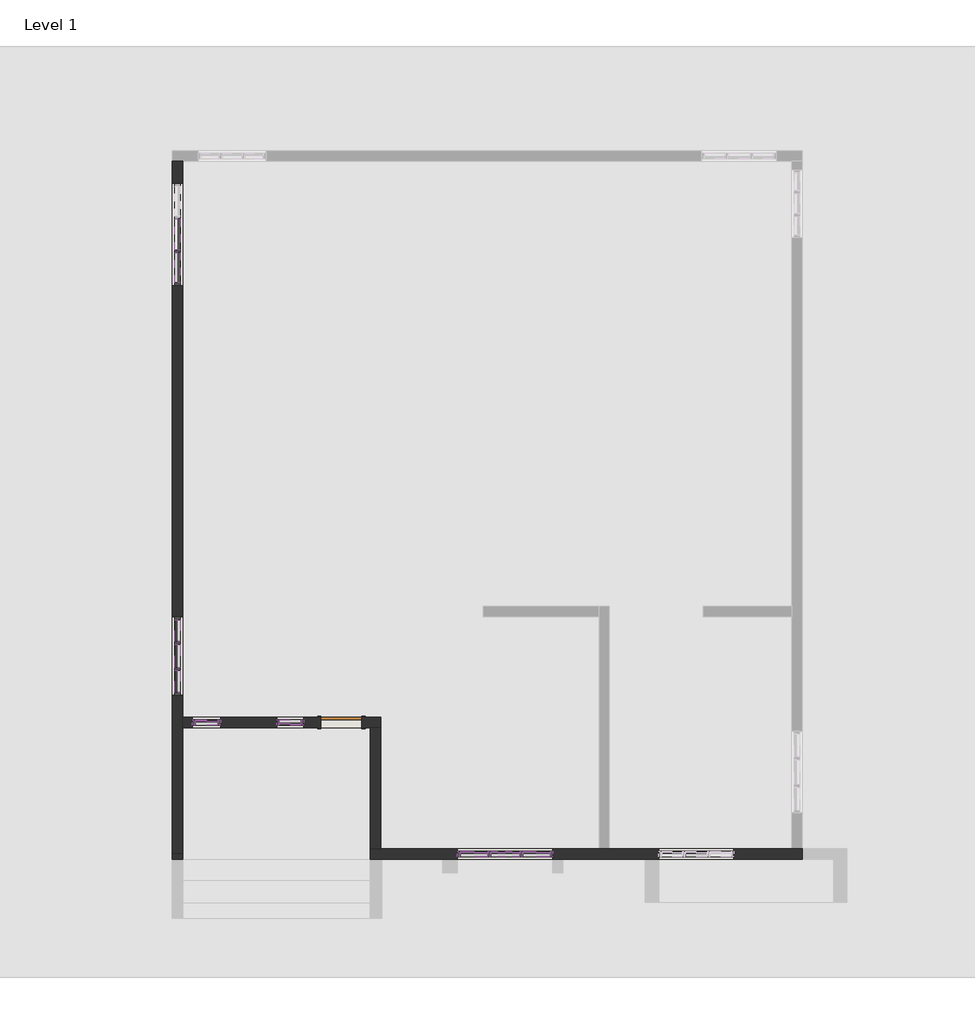
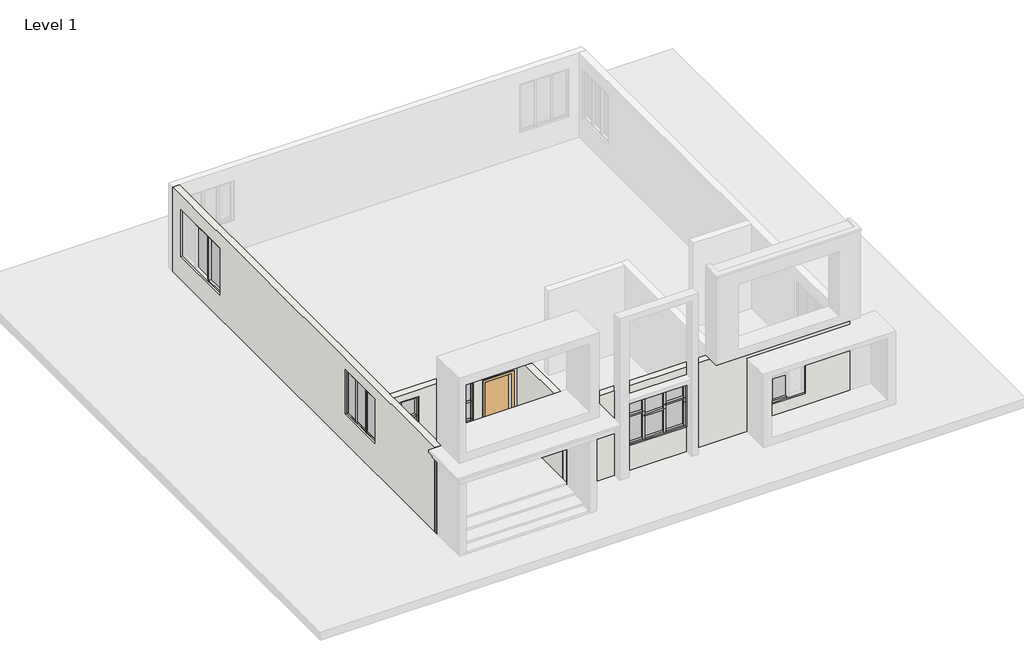
# One storey, part 1 of 2: 59 members, 19 plates, 5 walls, 1 door.
"""IFC4 building model written with IfcOpenShell, lengths in millimetres."""

from ifc_helpers import new_model, si_unit, origin, origin_with_axes, place, context, project, spatial, polyline, outline, extrude, faceted_brep, transform, mapped, element, save
from components import door_0ca8825f, member_5535eeb3, member_2ebf4a73, member_b955a9e9, member_c33c434a, member_d74592ed, member_67d70a96, member_b9f3750b, member_8f80d2aa, member_96e46165, member_de9b0c97, member_7fd687a9, member_90750a43, member_a9816f27, member_b70ee1cc, member_323df77c, member_86d06fe4, member_8600bbed, member_e53b78c9, member_5215b92c, member_3f0e0172, member_1cc7c027, member_f6f0dfdd, member_f8dc38bf, member_47c7a801, member_876f8f00, member_f09d9db7, member_ac493aea, member_2944fbe8, system_panel_glazed_7de79e50, system_panel_glazed_57682dc0, system_panel_glazed_8ac636d5, system_panel_glazed_c23b727d, system_panel_glazed_e55ceb02, system_panel_glazed_b26b014f, system_panel_glazed_bdd26bb3, system_panel_glazed_e612b4c2, system_panel_glazed_0ac8c76b, system_panel_glazed_a09e93fe, system_panel_glazed_b9962699, system_panel_glazed_c7c048a3, system_panel_glazed_0ee6699b, system_panel_glazed_40386fdd, system_panel_glazed_3330f8c4

model = new_model("IFC4")

# Units and contexts
model_context = context("Model", 3, world=origin())
ifc_project = project(units=[si_unit("LENGTHUNIT", "METRE", prefix="MILLI")], contexts=[model_context])

# Site, building, storey
site = spatial("IfcSite", under=ifc_project)
building = spatial("IfcBuilding", under=site)
storey = spatial("IfcBuildingStorey", under=building, Name="Level 1", Elevation=0.0)

# Door
placement = place(None, origin())
door_shape = door_0ca8825f(model_context)
element("IfcDoor", 1, ObjectType="Single-Flush : 36\" x 84\"", at=placement, inside=storey, context=model_context, shape_type="MappedRepresentation", body=[
    mapped(door_shape, transform((-18079.9097681, -11198.7339922, 406.4), x_axis=(1.0, 0.0, 0.0), y_axis=(0.0, 1.0, 0.0), z_axis=(0.0, 0.0, 1.0))),
])

# Members
member_shape = member_5535eeb3(model_context)
element("IfcMember", 2, ObjectType="Rectangular Mullion : 2.5\" x 5\" rectangular", at=placement, inside=storey, context=model_context, shape_type="MappedRepresentation", body=[
    mapped(member_shape, transform((-10466.2597681, -14132.4339922, 2463.7993261), x_axis=(0.0, 0.0, 1.0), y_axis=(0.0, -1.0, 0.0), z_axis=(1.0, 0.0, 0.0))),
])
member_2_shape = member_2ebf4a73(model_context)
element("IfcMember", 3, ObjectType="Rectangular Mullion : 2.5\" x 5\" rectangular", at=placement, inside=storey, context=model_context, shape_type="MappedRepresentation", body=[
    mapped(member_2_shape, transform((-10402.7597681, -14132.4339922, 684.1737808), x_axis=(0.0, 0.0, -1.0), y_axis=(0.0, -1.0, 0.0), z_axis=(-1.0, 0.0, 0.0))),
])
member_3_shape = member_b955a9e9(model_context)
element("IfcMember", 4, ObjectType="Rectangular Mullion : 2.5\" x 5\" rectangular", at=placement, inside=storey, context=model_context, shape_type="MappedRepresentation", body=[
    mapped(member_3_shape, transform((-21737.5097681, -651.3839922, 2530.4981779), x_axis=(0.0, 0.0, 1.0), y_axis=(-1.0, 0.0, 0.0), z_axis=(0.0, -1.0, 0.0))),
])
member_4_shape = member_c33c434a(model_context)
element("IfcMember", 5, ObjectType="Rectangular Mullion : 2.5\" x 5\" rectangular", at=placement, inside=storey, context=model_context, shape_type="MappedRepresentation", body=[
    mapped(member_4_shape, transform((-21737.5097681, -1381.6339922, 2530.4981779), x_axis=(0.0, 0.0, 1.0), y_axis=(-1.0, 0.0, 0.0), z_axis=(0.0, -1.0, 0.0))),
])
member_5_shape = member_d74592ed(model_context)
element("IfcMember", 6, ObjectType="Rectangular Mullion : 2.5\" x 5\" rectangular", at=placement, inside=storey, context=model_context, shape_type="MappedRepresentation", body=[
    mapped(member_5_shape, transform((-21737.5097681, -683.1339922, 850.000156), x_axis=(0.0, -1.0, 0.0), y_axis=(-1.0, 0.0, 0.0), z_axis=(0.0, 0.0, -1.0))),
])
element("IfcMember", 7, ObjectType="Rectangular Mullion : 2.5\" x 5\" rectangular", at=placement, inside=storey, context=model_context, shape_type="MappedRepresentation", body=[
    mapped(member_4_shape, transform((-21737.5097681, -714.8839922, 850.000156), x_axis=(0.0, 0.0, -1.0), y_axis=(-1.0, 0.0, 0.0), z_axis=(0.0, 1.0, 0.0))),
])
member_6_shape = member_67d70a96(model_context)
element("IfcMember", 8, ObjectType="Rectangular Mullion : 2.5\" x 5\" rectangular", at=placement, inside=storey, context=model_context, shape_type="MappedRepresentation", body=[
    mapped(member_6_shape, transform((-21737.5097681, -1445.1339922, 850.000156), x_axis=(0.0, -1.0, 0.0), y_axis=(-1.0, 0.0, 0.0), z_axis=(0.0, 0.0, -1.0))),
])
member_7_shape = member_b9f3750b(model_context)
element("IfcMember", 9, ObjectType="Rectangular Mullion : 2.5\" x 5\" rectangular", at=placement, inside=storey, context=model_context, shape_type="MappedRepresentation", body=[
    mapped(member_7_shape, transform((-21737.5097681, -10036.6839922, 2655.4428848), x_axis=(0.0, 0.0, 1.0), y_axis=(1.0, 0.0, 0.0), z_axis=(0.0, 1.0, 0.0))),
])
element("IfcMember", 10, ObjectType="Rectangular Mullion : 2.5\" x 5\" rectangular", at=placement, inside=storey, context=model_context, shape_type="MappedRepresentation", body=[
    mapped(member_7_shape, transform((-21737.5097681, -8900.0339922, 2655.4428848), x_axis=(0.0, 0.0, 1.0), y_axis=(1.0, 0.0, 0.0), z_axis=(0.0, 1.0, 0.0))),
])
member_8_shape = member_8f80d2aa(model_context)
element("IfcMember", 11, ObjectType="Rectangular Mullion : 2.5\" x 5\" rectangular", at=placement, inside=storey, context=model_context, shape_type="MappedRepresentation", body=[
    mapped(member_8_shape, transform((-21737.5097681, -9452.4839922, 2655.4428848), x_axis=(0.0, 0.0, 1.0), y_axis=(1.0, 0.0, 0.0), z_axis=(0.0, 1.0, 0.0))),
])
member_9_shape = member_96e46165(model_context)
element("IfcMember", 12, ObjectType="Rectangular Mullion : 2.5\" x 5\" rectangular", at=placement, inside=storey, context=model_context, shape_type="MappedRepresentation", body=[
    mapped(member_9_shape, transform((-21737.5097681, -9420.7339922, 1049.1745099), x_axis=(0.0, 1.0, 0.0), y_axis=(1.0, 0.0, 0.0), z_axis=(0.0, 0.0, -1.0))),
])
element("IfcMember", 13, ObjectType="Rectangular Mullion : 2.5\" x 5\" rectangular", at=placement, inside=storey, context=model_context, shape_type="MappedRepresentation", body=[
    mapped(member_9_shape, transform((-21737.5097681, -10004.9339922, 1049.1745099), x_axis=(0.0, 1.0, 0.0), y_axis=(1.0, 0.0, 0.0), z_axis=(0.0, 0.0, -1.0))),
])
element("IfcMember", 14, ObjectType="Rectangular Mullion : 2.5\" x 5\" rectangular", at=placement, inside=storey, context=model_context, shape_type="MappedRepresentation", body=[
    mapped(member_8_shape, transform((-21737.5097681, -9973.1839922, 1049.1745099), x_axis=(0.0, 0.0, -1.0), y_axis=(1.0, 0.0, 0.0), z_axis=(0.0, -1.0, 0.0))),
])
element("IfcMember", 15, ObjectType="Rectangular Mullion : 2.5\" x 5\" rectangular", at=placement, inside=storey, context=model_context, shape_type="MappedRepresentation", body=[
    mapped(member_7_shape, transform((-21737.5097681, -9388.9839922, 1049.1745099), x_axis=(0.0, 0.0, -1.0), y_axis=(1.0, 0.0, 0.0), z_axis=(0.0, -1.0, 0.0))),
])
element("IfcMember", 16, ObjectType="Rectangular Mullion : 2.5\" x 5\" rectangular", at=placement, inside=storey, context=model_context, shape_type="MappedRepresentation", body=[
    mapped(member_7_shape, transform((-21737.5097681, -10525.6339922, 1049.1745099), x_axis=(0.0, 0.0, -1.0), y_axis=(1.0, 0.0, 0.0), z_axis=(0.0, -1.0, 0.0))),
])
member_10_shape = member_de9b0c97(model_context)
element("IfcMember", 17, ObjectType="Rectangular Mullion : 2.5\" x 5\" rectangular", at=placement, inside=storey, context=model_context, shape_type="MappedRepresentation", body=[
    mapped(member_10_shape, transform((-21737.5097681, -10589.1339922, 2655.4428848), x_axis=(0.0, -1.0, 0.0), y_axis=(1.0, 0.0, 0.0), z_axis=(0.0, 0.0, 1.0))),
])
element("IfcMember", 18, ObjectType="Rectangular Mullion : 2.5\" x 5\" rectangular", at=placement, inside=storey, context=model_context, shape_type="MappedRepresentation", body=[
    mapped(member_10_shape, transform((-21737.5097681, -8836.5339922, 1049.1745099), x_axis=(0.0, 1.0, 0.0), y_axis=(1.0, 0.0, 0.0), z_axis=(0.0, 0.0, -1.0))),
])
member_11_shape = member_7fd687a9(model_context)
element("IfcMember", 19, ObjectType="Rectangular Mullion : 2.5\" x 5\" rectangular", at=placement, inside=storey, context=model_context, shape_type="MappedRepresentation", body=[
    mapped(member_11_shape, transform((-20835.8097681, -11198.7339922, 2808.8134726), x_axis=(0.0, 0.0, 1.0), y_axis=(0.0, -1.0, 0.0), z_axis=(1.0, 0.0, 0.0))),
])
member_12_shape = member_90750a43(model_context)
element("IfcMember", 20, ObjectType="Rectangular Mullion : 2.5\" x 5\" rectangular", at=placement, inside=storey, context=model_context, shape_type="MappedRepresentation", body=[
    mapped(member_12_shape, transform((-20835.8097681, -11198.7339922, 2112.2396553), x_axis=(0.0, 0.0, 1.0), y_axis=(0.0, -1.0, 0.0), z_axis=(1.0, 0.0, 0.0))),
])
element("IfcMember", 21, ObjectType="Rectangular Mullion : 2.5\" x 5\" rectangular", at=placement, inside=storey, context=model_context, shape_type="MappedRepresentation", body=[
    mapped(member_12_shape, transform((-20835.8097681, -11198.7339922, 1415.6658381), x_axis=(0.0, 0.0, 1.0), y_axis=(0.0, -1.0, 0.0), z_axis=(1.0, 0.0, 0.0))),
])
member_13_shape = member_a9816f27(model_context)
element("IfcMember", 22, ObjectType="Rectangular Mullion : 2.5\" x 5\" rectangular", at=placement, inside=storey, context=model_context, shape_type="MappedRepresentation", body=[
    mapped(member_13_shape, transform((-20772.3097681, -11198.7339922, 2112.2396553), x_axis=(1.0, 0.0, 0.0), y_axis=(0.0, -1.0, 0.0), z_axis=(0.0, 0.0, -1.0))),
])
element("IfcMember", 23, ObjectType="Rectangular Mullion : 2.5\" x 5\" rectangular", at=placement, inside=storey, context=model_context, shape_type="MappedRepresentation", body=[
    mapped(member_13_shape, transform((-21407.3097681, -11198.7339922, 2808.8134726), x_axis=(-1.0, 0.0, 0.0), y_axis=(0.0, -1.0, 0.0), z_axis=(0.0, 0.0, 1.0))),
])
element("IfcMember", 24, ObjectType="Rectangular Mullion : 2.5\" x 5\" rectangular", at=placement, inside=storey, context=model_context, shape_type="MappedRepresentation", body=[
    mapped(member_13_shape, transform((-20772.3097681, -11198.7339922, 1415.6658381), x_axis=(1.0, 0.0, 0.0), y_axis=(0.0, -1.0, 0.0), z_axis=(0.0, 0.0, -1.0))),
])
element("IfcMember", 25, ObjectType="Rectangular Mullion : 2.5\" x 5\" rectangular", at=placement, inside=storey, context=model_context, shape_type="MappedRepresentation", body=[
    mapped(member_13_shape, transform((-21407.3097681, -11198.7339922, 2112.2396553), x_axis=(-1.0, 0.0, 0.0), y_axis=(0.0, -1.0, 0.0), z_axis=(0.0, 0.0, 1.0))),
])
element("IfcMember", 26, ObjectType="Rectangular Mullion : 2.5\" x 5\" rectangular", at=placement, inside=storey, context=model_context, shape_type="MappedRepresentation", body=[
    mapped(member_11_shape, transform((-21343.8097681, -11198.7339922, 719.0920209), x_axis=(0.0, 0.0, -1.0), y_axis=(0.0, -1.0, 0.0), z_axis=(-1.0, 0.0, 0.0))),
])
element("IfcMember", 27, ObjectType="Rectangular Mullion : 2.5\" x 5\" rectangular", at=placement, inside=storey, context=model_context, shape_type="MappedRepresentation", body=[
    mapped(member_13_shape, transform((-20772.3097681, -11198.7339922, 719.0920209), x_axis=(1.0, 0.0, 0.0), y_axis=(0.0, -1.0, 0.0), z_axis=(0.0, 0.0, -1.0))),
])
element("IfcMember", 28, ObjectType="Rectangular Mullion : 2.5\" x 5\" rectangular", at=placement, inside=storey, context=model_context, shape_type="MappedRepresentation", body=[
    mapped(member_13_shape, transform((-21407.3097681, -11198.7339922, 1415.6658381), x_axis=(-1.0, 0.0, 0.0), y_axis=(0.0, -1.0, 0.0), z_axis=(0.0, 0.0, 1.0))),
])
member_14_shape = member_b70ee1cc(model_context)
element("IfcMember", 29, ObjectType="Rectangular Mullion : 2.5\" x 5\" rectangular", at=placement, inside=storey, context=model_context, shape_type="MappedRepresentation", body=[
    mapped(member_14_shape, transform((-19527.7097681, -11198.7339922, 1978.8215035), x_axis=(-1.0, 0.0, 0.0), y_axis=(0.0, 1.0, 0.0), z_axis=(0.0, 0.0, -1.0))),
])
member_15_shape = member_323df77c(model_context)
element("IfcMember", 30, ObjectType="Rectangular Mullion : 2.5\" x 5\" rectangular", at=placement, inside=storey, context=model_context, shape_type="MappedRepresentation", body=[
    mapped(member_15_shape, transform((-19464.2097681, -11198.7339922, 1978.8215035), x_axis=(0.0, 0.0, 1.0), y_axis=(0.0, 1.0, 0.0), z_axis=(-1.0, 0.0, 0.0))),
])
element("IfcMember", 31, ObjectType="Rectangular Mullion : 2.5\" x 5\" rectangular", at=placement, inside=storey, context=model_context, shape_type="MappedRepresentation", body=[
    mapped(member_15_shape, transform((-19464.2097681, -11198.7339922, 1330.4078609), x_axis=(0.0, 0.0, 1.0), y_axis=(0.0, 1.0, 0.0), z_axis=(-1.0, 0.0, 0.0))),
])
member_16_shape = member_86d06fe4(model_context)
element("IfcMember", 32, ObjectType="Rectangular Mullion : 2.5\" x 5\" rectangular", at=placement, inside=storey, context=model_context, shape_type="MappedRepresentation", body=[
    mapped(member_16_shape, transform((-19464.2097681, -11198.7339922, 2842.4215035), x_axis=(0.0, 0.0, 1.0), y_axis=(0.0, 1.0, 0.0), z_axis=(-1.0, 0.0, 0.0))),
])
element("IfcMember", 33, ObjectType="Rectangular Mullion : 2.5\" x 5\" rectangular", at=placement, inside=storey, context=model_context, shape_type="MappedRepresentation", body=[
    mapped(member_14_shape, transform((-18918.1097681, -11198.7339922, 2842.4215035), x_axis=(1.0, 0.0, 0.0), y_axis=(0.0, 1.0, 0.0), z_axis=(0.0, 0.0, 1.0))),
])
element("IfcMember", 34, ObjectType="Rectangular Mullion : 2.5\" x 5\" rectangular", at=placement, inside=storey, context=model_context, shape_type="MappedRepresentation", body=[
    mapped(member_16_shape, transform((-18981.6097681, -11198.7339922, 681.9942183), x_axis=(0.0, 0.0, -1.0), y_axis=(0.0, 1.0, 0.0), z_axis=(1.0, 0.0, 0.0))),
])
member_17_shape = member_8600bbed(model_context)
element("IfcMember", 35, ObjectType="Rectangular Mullion : 2.5\" x 5\" rectangular", at=placement, inside=storey, context=model_context, shape_type="MappedRepresentation", body=[
    mapped(member_17_shape, transform((-19527.7097681, -11198.7339922, 1330.4078609), x_axis=(-1.0, 0.0, 0.0), y_axis=(0.0, 1.0, 0.0), z_axis=(0.0, 0.0, -1.0))),
])
element("IfcMember", 36, ObjectType="Rectangular Mullion : 2.5\" x 5\" rectangular", at=placement, inside=storey, context=model_context, shape_type="MappedRepresentation", body=[
    mapped(member_17_shape, transform((-19527.7097681, -11198.7339922, 681.9942183), x_axis=(-1.0, 0.0, 0.0), y_axis=(0.0, 1.0, 0.0), z_axis=(0.0, 0.0, -1.0))),
])
element("IfcMember", 37, ObjectType="Rectangular Mullion : 2.5\" x 5\" rectangular", at=placement, inside=storey, context=model_context, shape_type="MappedRepresentation", body=[
    mapped(member_17_shape, transform((-18918.1097681, -11198.7339922, 1330.4078609), x_axis=(1.0, 0.0, 0.0), y_axis=(0.0, 1.0, 0.0), z_axis=(0.0, 0.0, 1.0))),
])
element("IfcMember", 38, ObjectType="Rectangular Mullion : 2.5\" x 5\" rectangular", at=placement, inside=storey, context=model_context, shape_type="MappedRepresentation", body=[
    mapped(member_17_shape, transform((-18918.1097681, -11198.7339922, 1978.8215035), x_axis=(1.0, 0.0, 0.0), y_axis=(0.0, 1.0, 0.0), z_axis=(0.0, 0.0, 1.0))),
])
member_18_shape = member_e53b78c9(model_context)
element("IfcMember", 39, ObjectType="Rectangular Mullion : 2.5\" x 5\" rectangular", at=placement, inside=storey, context=model_context, shape_type="MappedRepresentation", body=[
    mapped(member_18_shape, transform((-14098.4597681, -14132.4339922, 1762.5660143), x_axis=(0.0, 0.0, 1.0), y_axis=(0.0, -1.0, 0.0), z_axis=(1.0, 0.0, 0.0))),
])
member_19_shape = member_5215b92c(model_context)
element("IfcMember", 40, ObjectType="Rectangular Mullion : 2.5\" x 5\" rectangular", at=placement, inside=storey, context=model_context, shape_type="MappedRepresentation", body=[
    mapped(member_19_shape, transform((-14098.4597681, -14132.4339922, 2636.1562178), x_axis=(0.0, 0.0, 1.0), y_axis=(0.0, -1.0, 0.0), z_axis=(1.0, 0.0, 0.0))),
])
member_20_shape = member_3f0e0172(model_context)
element("IfcMember", 41, ObjectType="Rectangular Mullion : 2.5\" x 5\" rectangular", at=placement, inside=storey, context=model_context, shape_type="MappedRepresentation", body=[
    mapped(member_20_shape, transform((-14809.6597681, -14132.4339922, 2636.1562178), x_axis=(0.0, 0.0, 1.0), y_axis=(0.0, -1.0, 0.0), z_axis=(1.0, 0.0, 0.0))),
])
element("IfcMember", 42, ObjectType="Rectangular Mullion : 2.5\" x 5\" rectangular", at=placement, inside=storey, context=model_context, shape_type="MappedRepresentation", body=[
    mapped(member_20_shape, transform((-13419.0097681, -14132.4339922, 2636.1562178), x_axis=(0.0, 0.0, 1.0), y_axis=(0.0, -1.0, 0.0), z_axis=(1.0, 0.0, 0.0))),
])
member_21_shape = member_1cc7c027(model_context)
element("IfcMember", 43, ObjectType="Rectangular Mullion : 2.5\" x 5\" rectangular", at=placement, inside=storey, context=model_context, shape_type="MappedRepresentation", body=[
    mapped(member_21_shape, transform((-14777.9097681, -14132.4339922, 1914.9660143), x_axis=(1.0, 0.0, 0.0), y_axis=(0.0, -1.0, 0.0), z_axis=(0.0, 0.0, -1.0))),
])
element("IfcMember", 44, ObjectType="Rectangular Mullion : 2.5\" x 5\" rectangular", at=placement, inside=storey, context=model_context, shape_type="MappedRepresentation", body=[
    mapped(member_21_shape, transform((-14066.7097681, -14132.4339922, 1914.9660143), x_axis=(1.0, 0.0, 0.0), y_axis=(0.0, -1.0, 0.0), z_axis=(0.0, 0.0, -1.0))),
])
member_22_shape = member_f6f0dfdd(model_context)
element("IfcMember", 45, ObjectType="Rectangular Mullion : 2.5\" x 5\" rectangular", at=placement, inside=storey, context=model_context, shape_type="MappedRepresentation", body=[
    mapped(member_22_shape, transform((-14777.9097681, -14132.4339922, 1762.5660143), x_axis=(1.0, 0.0, 0.0), y_axis=(0.0, -1.0, 0.0), z_axis=(0.0, 0.0, -1.0))),
])
element("IfcMember", 46, ObjectType="Rectangular Mullion : 2.5\" x 5\" rectangular", at=placement, inside=storey, context=model_context, shape_type="MappedRepresentation", body=[
    mapped(member_22_shape, transform((-14066.7097681, -14132.4339922, 1762.5660143), x_axis=(1.0, 0.0, 0.0), y_axis=(0.0, -1.0, 0.0), z_axis=(0.0, 0.0, -1.0))),
])
member_23_shape = member_f8dc38bf(model_context)
element("IfcMember", 47, ObjectType="Rectangular Mullion : 2.5\" x 5\" rectangular", at=placement, inside=storey, context=model_context, shape_type="MappedRepresentation", body=[
    mapped(member_23_shape, transform((-13419.0097681, -14132.4339922, 1914.9660143), x_axis=(0.0, 0.0, 1.0), y_axis=(0.0, -1.0, 0.0), z_axis=(1.0, 0.0, 0.0))),
])
element("IfcMember", 48, ObjectType="Rectangular Mullion : 2.5\" x 5\" rectangular", at=placement, inside=storey, context=model_context, shape_type="MappedRepresentation", body=[
    mapped(member_23_shape, transform((-14809.6597681, -14132.4339922, 1914.9660143), x_axis=(0.0, 0.0, 1.0), y_axis=(0.0, -1.0, 0.0), z_axis=(1.0, 0.0, 0.0))),
])
member_24_shape = member_47c7a801(model_context)
element("IfcMember", 49, ObjectType="Rectangular Mullion : 2.5\" x 5\" rectangular", at=placement, inside=storey, context=model_context, shape_type="MappedRepresentation", body=[
    mapped(member_24_shape, transform((-13355.5097681, -14132.4339922, 1914.9660143), x_axis=(1.0, 0.0, 0.0), y_axis=(0.0, -1.0, 0.0), z_axis=(0.0, 0.0, -1.0))),
])
member_25_shape = member_876f8f00(model_context)
element("IfcMember", 50, ObjectType="Rectangular Mullion : 2.5\" x 5\" rectangular", at=placement, inside=storey, context=model_context, shape_type="MappedRepresentation", body=[
    mapped(member_25_shape, transform((-13355.5097681, -14132.4339922, 1762.5660143), x_axis=(1.0, 0.0, 0.0), y_axis=(0.0, -1.0, 0.0), z_axis=(0.0, 0.0, -1.0))),
])
element("IfcMember", 51, ObjectType="Rectangular Mullion : 2.5\" x 5\" rectangular", at=placement, inside=storey, context=model_context, shape_type="MappedRepresentation", body=[
    mapped(member_25_shape, transform((-15489.1097681, -14132.4339922, 1914.9660143), x_axis=(-1.0, 0.0, 0.0), y_axis=(0.0, -1.0, 0.0), z_axis=(0.0, 0.0, 1.0))),
])
element("IfcMember", 52, ObjectType="Rectangular Mullion : 2.5\" x 5\" rectangular", at=placement, inside=storey, context=model_context, shape_type="MappedRepresentation", body=[
    mapped(member_24_shape, transform((-15489.1097681, -14132.4339922, 2636.1562178), x_axis=(-1.0, 0.0, 0.0), y_axis=(0.0, -1.0, 0.0), z_axis=(0.0, 0.0, 1.0))),
])
member_26_shape = member_f09d9db7(model_context)
element("IfcMember", 53, ObjectType="Rectangular Mullion : 2.5\" x 5\" rectangular", at=placement, inside=storey, context=model_context, shape_type="MappedRepresentation", body=[
    mapped(member_26_shape, transform((-14777.9097681, -14132.4339922, 888.9758108), x_axis=(1.0, 0.0, 0.0), y_axis=(0.0, -1.0, 0.0), z_axis=(0.0, 0.0, -1.0))),
])
element("IfcMember", 54, ObjectType="Rectangular Mullion : 2.5\" x 5\" rectangular", at=placement, inside=storey, context=model_context, shape_type="MappedRepresentation", body=[
    mapped(member_26_shape, transform((-14066.7097681, -14132.4339922, 888.9758108), x_axis=(1.0, 0.0, 0.0), y_axis=(0.0, -1.0, 0.0), z_axis=(0.0, 0.0, -1.0))),
])
element("IfcMember", 55, ObjectType="Rectangular Mullion : 2.5\" x 5\" rectangular", at=placement, inside=storey, context=model_context, shape_type="MappedRepresentation", body=[
    mapped(member_20_shape, transform((-14034.9597681, -14132.4339922, 888.9758108), x_axis=(0.0, 0.0, -1.0), y_axis=(0.0, -1.0, 0.0), z_axis=(-1.0, 0.0, 0.0))),
])
element("IfcMember", 56, ObjectType="Rectangular Mullion : 2.5\" x 5\" rectangular", at=placement, inside=storey, context=model_context, shape_type="MappedRepresentation", body=[
    mapped(member_20_shape, transform((-15425.6097681, -14132.4339922, 888.9758108), x_axis=(0.0, 0.0, -1.0), y_axis=(0.0, -1.0, 0.0), z_axis=(-1.0, 0.0, 0.0))),
])
element("IfcMember", 57, ObjectType="Rectangular Mullion : 2.5\" x 5\" rectangular", at=placement, inside=storey, context=model_context, shape_type="MappedRepresentation", body=[
    mapped(member_19_shape, transform((-14746.1597681, -14132.4339922, 888.9758108), x_axis=(0.0, 0.0, -1.0), y_axis=(0.0, -1.0, 0.0), z_axis=(-1.0, 0.0, 0.0))),
])
member_27_shape = member_ac493aea(model_context)
element("IfcMember", 58, ObjectType="Rectangular Mullion : 2.5\" x 5\" rectangular", at=placement, inside=storey, context=model_context, shape_type="MappedRepresentation", body=[
    mapped(member_27_shape, transform((-13355.5097681, -14132.4339922, 888.9758108), x_axis=(1.0, 0.0, 0.0), y_axis=(0.0, -1.0, 0.0), z_axis=(0.0, 0.0, -1.0))),
])
element("IfcMember", 59, ObjectType="Rectangular Mullion : 2.5\" x 5\" rectangular", at=placement, inside=storey, context=model_context, shape_type="MappedRepresentation", body=[
    mapped(member_27_shape, transform((-15489.1097681, -14132.4339922, 1762.5660143), x_axis=(-1.0, 0.0, 0.0), y_axis=(0.0, -1.0, 0.0), z_axis=(0.0, 0.0, 1.0))),
])
member_28_shape = member_2944fbe8(model_context)
element("IfcMember", 60, ObjectType="Rectangular Mullion : 2.5\" x 5\" rectangular", at=placement, inside=storey, context=model_context, shape_type="MappedRepresentation", body=[
    mapped(member_28_shape, transform((-10993.3097681, -14132.4339922, 2463.7993261), x_axis=(-1.0, 0.0, 0.0), y_axis=(0.0, -1.0, 0.0), z_axis=(0.0, 0.0, 1.0))),
])

# Plates
system_panel_glazed_shape = system_panel_glazed_7de79e50(model_context)
element("IfcPlate", 61, ObjectType="System Panel : Glazed", at=placement, inside=storey, context=model_context, shape_type="MappedRepresentation", body=[
    mapped(system_panel_glazed_shape, transform((-21737.5097681, -1048.2589922, 913.500156), x_axis=(0.0, -1.0, 0.0), y_axis=(1.0, 0.0, 0.0), z_axis=(0.0, 0.0, 1.0))),
])
system_panel_glazed_2_shape = system_panel_glazed_57682dc0(model_context)
element("IfcPlate", 62, ObjectType="System Panel : Glazed", at=placement, inside=storey, context=model_context, shape_type="MappedRepresentation", body=[
    mapped(system_panel_glazed_2_shape, transform((-21737.5097681, -302.1339922, 913.500156), x_axis=(0.0, -1.0, 0.0), y_axis=(1.0, 0.0, 0.0), z_axis=(0.0, 0.0, 1.0))),
])
system_panel_glazed_3_shape = system_panel_glazed_8ac636d5(model_context)
element("IfcPlate", 63, ObjectType="System Panel : Glazed", at=placement, inside=storey, context=model_context, shape_type="MappedRepresentation", body=[
    mapped(system_panel_glazed_3_shape, transform((-21737.5097681, -10281.1589922, 1112.6745099), x_axis=(0.0, 1.0, 0.0), y_axis=(-1.0, 0.0, 0.0), z_axis=(0.0, 0.0, 1.0))),
])
element("IfcPlate", 64, ObjectType="System Panel : Glazed", at=placement, inside=storey, context=model_context, shape_type="MappedRepresentation", body=[
    mapped(system_panel_glazed_3_shape, transform((-21737.5097681, -9144.5089922, 1112.6745099), x_axis=(0.0, 1.0, 0.0), y_axis=(-1.0, 0.0, 0.0), z_axis=(0.0, 0.0, 1.0))),
])
system_panel_glazed_4_shape = system_panel_glazed_c23b727d(model_context)
element("IfcPlate", 65, ObjectType="System Panel : Glazed", at=placement, inside=storey, context=model_context, shape_type="MappedRepresentation", body=[
    mapped(system_panel_glazed_4_shape, transform((-21737.5097681, -9712.8339922, 1112.6745099), x_axis=(0.0, 1.0, 0.0), y_axis=(-1.0, 0.0, 0.0), z_axis=(0.0, 0.0, 1.0))),
])
system_panel_glazed_5_shape = system_panel_glazed_e55ceb02(model_context)
element("IfcPlate", 66, ObjectType="System Panel : Glazed", at=placement, inside=storey, context=model_context, shape_type="MappedRepresentation", body=[
    mapped(system_panel_glazed_5_shape, transform((-21089.8097681, -11198.7339922, 782.5920209), x_axis=(1.0, 0.0, 0.0), y_axis=(0.0, 1.0, 0.0), z_axis=(0.0, 0.0, 1.0))),
])
element("IfcPlate", 67, ObjectType="System Panel : Glazed", at=placement, inside=storey, context=model_context, shape_type="MappedRepresentation", body=[
    mapped(system_panel_glazed_5_shape, transform((-21089.8097681, -11198.7339922, 2143.9896553), x_axis=(1.0, 0.0, 0.0), y_axis=(0.0, 1.0, 0.0), z_axis=(0.0, 0.0, 1.0))),
])
system_panel_glazed_6_shape = system_panel_glazed_b26b014f(model_context)
element("IfcPlate", 68, ObjectType="System Panel : Glazed", at=placement, inside=storey, context=model_context, shape_type="MappedRepresentation", body=[
    mapped(system_panel_glazed_6_shape, transform((-21089.8097681, -11198.7339922, 1447.4158381), x_axis=(1.0, 0.0, 0.0), y_axis=(0.0, 1.0, 0.0), z_axis=(0.0, 0.0, 1.0))),
])
system_panel_glazed_7_shape = system_panel_glazed_bdd26bb3(model_context)
element("IfcPlate", 69, ObjectType="System Panel : Glazed", at=placement, inside=storey, context=model_context, shape_type="MappedRepresentation", body=[
    mapped(system_panel_glazed_7_shape, transform((-19222.9097681, -11198.7339922, 2010.5715035), x_axis=(-1.0, 0.0, 0.0), y_axis=(0.0, -1.0, 0.0), z_axis=(0.0, 0.0, 1.0))),
])
system_panel_glazed_8_shape = system_panel_glazed_e612b4c2(model_context)
element("IfcPlate", 70, ObjectType="System Panel : Glazed", at=placement, inside=storey, context=model_context, shape_type="MappedRepresentation", body=[
    mapped(system_panel_glazed_8_shape, transform((-19222.9097681, -11198.7339922, 1362.1578609), x_axis=(-1.0, 0.0, 0.0), y_axis=(0.0, -1.0, 0.0), z_axis=(0.0, 0.0, 1.0))),
])
system_panel_glazed_9_shape = system_panel_glazed_0ac8c76b(model_context)
element("IfcPlate", 71, ObjectType="System Panel : Glazed", at=placement, inside=storey, context=model_context, shape_type="MappedRepresentation", body=[
    mapped(system_panel_glazed_9_shape, transform((-19222.9097681, -11198.7339922, 745.4942183), x_axis=(-1.0, 0.0, 0.0), y_axis=(0.0, -1.0, 0.0), z_axis=(0.0, 0.0, 1.0))),
])
system_panel_glazed_10_shape = system_panel_glazed_a09e93fe(model_context)
element("IfcPlate", 72, ObjectType="System Panel : Glazed", at=placement, inside=storey, context=model_context, shape_type="MappedRepresentation", body=[
    mapped(system_panel_glazed_10_shape, transform((-14422.3097681, -14132.4339922, 1794.3160143), x_axis=(1.0, 0.0, 0.0), y_axis=(0.0, 1.0, 0.0), z_axis=(0.0, 0.0, 1.0))),
])
system_panel_glazed_11_shape = system_panel_glazed_b9962699(model_context)
element("IfcPlate", 73, ObjectType="System Panel : Glazed", at=placement, inside=storey, context=model_context, shape_type="MappedRepresentation", body=[
    mapped(system_panel_glazed_11_shape, transform((-15117.6347681, -14132.4339922, 1946.7160143), x_axis=(1.0, 0.0, 0.0), y_axis=(0.0, 1.0, 0.0), z_axis=(0.0, 0.0, 1.0))),
])
element("IfcPlate", 74, ObjectType="System Panel : Glazed", at=placement, inside=storey, context=model_context, shape_type="MappedRepresentation", body=[
    mapped(system_panel_glazed_11_shape, transform((-13726.9847681, -14132.4339922, 1946.7160143), x_axis=(1.0, 0.0, 0.0), y_axis=(0.0, 1.0, 0.0), z_axis=(0.0, 0.0, 1.0))),
])
system_panel_glazed_12_shape = system_panel_glazed_c7c048a3(model_context)
element("IfcPlate", 75, ObjectType="System Panel : Glazed", at=placement, inside=storey, context=model_context, shape_type="MappedRepresentation", body=[
    mapped(system_panel_glazed_12_shape, transform((-15117.6347681, -14132.4339922, 952.4758108), x_axis=(1.0, 0.0, 0.0), y_axis=(0.0, 1.0, 0.0), z_axis=(0.0, 0.0, 1.0))),
])
element("IfcPlate", 76, ObjectType="System Panel : Glazed", at=placement, inside=storey, context=model_context, shape_type="MappedRepresentation", body=[
    mapped(system_panel_glazed_12_shape, transform((-13726.9847681, -14132.4339922, 952.4758108), x_axis=(1.0, 0.0, 0.0), y_axis=(0.0, 1.0, 0.0), z_axis=(0.0, 0.0, 1.0))),
])
system_panel_glazed_13_shape = system_panel_glazed_0ee6699b(model_context)
element("IfcPlate", 77, ObjectType="System Panel : Glazed", at=placement, inside=storey, context=model_context, shape_type="MappedRepresentation", body=[
    mapped(system_panel_glazed_13_shape, transform((-14422.3097681, -14132.4339922, 952.4758108), x_axis=(1.0, 0.0, 0.0), y_axis=(0.0, 1.0, 0.0), z_axis=(0.0, 0.0, 1.0))),
])
system_panel_glazed_14_shape = system_panel_glazed_40386fdd(model_context)
element("IfcPlate", 78, ObjectType="System Panel : Glazed", at=placement, inside=storey, context=model_context, shape_type="MappedRepresentation", body=[
    mapped(system_panel_glazed_14_shape, transform((-10698.0347681, -14132.4339922, 747.6737808), x_axis=(1.0, 0.0, 0.0), y_axis=(0.0, 1.0, 0.0), z_axis=(0.0, 0.0, 1.0))),
])
system_panel_glazed_15_shape = system_panel_glazed_3330f8c4(model_context)
element("IfcPlate", 79, ObjectType="System Panel : Glazed", at=placement, inside=storey, context=model_context, shape_type="MappedRepresentation", body=[
    mapped(system_panel_glazed_15_shape, transform((-10155.1097681, -14132.4339922, 747.6737808), x_axis=(1.0, 0.0, 0.0), y_axis=(0.0, 1.0, 0.0), z_axis=(0.0, 0.0, 1.0))),
])

# Walls
element("IfcWall", 80, ObjectType="9\"", at=placement, inside=storey, context=model_context, shape_type="Brep", body=[
    faceted_brep([(-21851.8097681, 1336.1660078, 0.0), (-21851.8097681, -14132.4339922, 0.0), (-21851.8097681, -14132.4339922, 3048.0), (-21851.8097681, 1336.1660078, 3048.0), (-21851.8097681, 840.8660078, 850.000156), (-21851.8097681, 840.8660078, 2530.4981779), (-21851.8097681, -1445.1339922, 2530.4981779), (-21851.8097681, -1445.1339922, 850.000156), (-21851.8097681, -10589.1339922, 2655.4428848), (-21851.8097681, -10589.1339922, 1049.1745099), (-21851.8097681, -8836.5339922, 1049.1745099), (-21851.8097681, -8836.5339922, 2655.4428848), (-21623.2097681, -14132.4339922, 0.0), (-21623.2097681, -11313.0339922, 0.0), (-21623.2097681, -11084.4339922, 0.0), (-21623.2097681, 1336.1660078, 0.0), (-21623.2097681, 1336.1660078, 3048.0), (-21623.2097681, -11084.4339922, 3048.0), (-21623.2097681, -11313.0339922, 3048.0), (-21623.2097681, -14132.4339922, 3048.0), (-21623.2097681, 840.8660078, 2530.4981779), (-21623.2097681, 840.8660078, 850.000156), (-21623.2097681, -1445.1339922, 850.000156), (-21623.2097681, -1445.1339922, 2530.4981779), (-21623.2097681, -10589.1339922, 1049.1745099), (-21623.2097681, -10589.1339922, 2655.4428848), (-21623.2097681, -8836.5339922, 2655.4428848), (-21623.2097681, -8836.5339922, 1049.1745099)], [[[0, 1, 2, 3], [4, 5, 6, 7], [8, 9, 10, 11]], [[12, 13, 14, 15, 16, 17, 18, 19], [20, 21, 22, 23], [24, 25, 26, 27]], [[1, 0, 15, 14, 13, 12]], [[2, 1, 12, 19]], [[3, 2, 19, 18, 17, 16]], [[0, 3, 16, 15]], [[4, 21, 20, 5]], [[5, 20, 23, 6]], [[6, 23, 22, 7]], [[21, 4, 7, 22]], [[24, 9, 8, 25]], [[25, 8, 11, 26]], [[10, 27, 26, 11]], [[9, 24, 27, 10]]]),
])
element("IfcWall", 81, ObjectType="9\"", at=placement, inside=storey, context=model_context, shape_type="Brep", body=[
    faceted_brep([(-21623.2097681, -11313.0339922, 0.0), (-17432.2097681, -11313.0339922, 0.0), (-17203.6097681, -11313.0339922, 0.0), (-17203.6097681, -11313.0339922, 3048.0), (-17432.2097681, -11313.0339922, 3048.0), (-21623.2097681, -11313.0339922, 3048.0), (-17622.7097681, -11313.0339922, 406.4), (-18537.1097681, -11313.0339922, 406.4), (-18537.1097681, -11313.0339922, 2540.0), (-17622.7097681, -11313.0339922, 2540.0), (-21407.3097681, -11313.0339922, 719.0920209), (-21407.3097681, -11313.0339922, 2808.8134726), (-20772.3097681, -11313.0339922, 2808.8134726), (-20772.3097681, -11313.0339922, 719.0920209), (-18918.1097681, -11313.0339922, 2842.4215035), (-18918.1097681, -11313.0339922, 681.9942183), (-19527.7097681, -11313.0339922, 681.9942183), (-19527.7097681, -11313.0339922, 2842.4215035), (-17203.6097681, -11084.4339922, 0.0), (-21623.2097681, -11084.4339922, 0.0), (-21623.2097681, -11084.4339922, 3048.0), (-17203.6097681, -11084.4339922, 3048.0), (-18537.1097681, -11084.4339922, 406.4), (-17622.7097681, -11084.4339922, 406.4), (-17622.7097681, -11084.4339922, 2540.0), (-18537.1097681, -11084.4339922, 2540.0), (-21407.3097681, -11084.4339922, 2808.8134726), (-21407.3097681, -11084.4339922, 719.0920209), (-20772.3097681, -11084.4339922, 719.0920209), (-20772.3097681, -11084.4339922, 2808.8134726), (-18918.1097681, -11084.4339922, 681.9942183), (-18918.1097681, -11084.4339922, 2842.4215035), (-19527.7097681, -11084.4339922, 2842.4215035), (-19527.7097681, -11084.4339922, 681.9942183)], [[[0, 1, 2, 3, 4, 5], [6, 7, 8, 9], [10, 11, 12, 13], [14, 15, 16, 17]], [[18, 19, 20, 21], [22, 23, 24, 25], [26, 27, 28, 29], [30, 31, 32, 33]], [[2, 1, 0, 19, 18]], [[5, 4, 3, 21, 20]], [[0, 5, 20, 19]], [[3, 2, 18, 21]], [[23, 22, 7, 6]], [[24, 23, 6, 9]], [[25, 24, 9, 8]], [[22, 25, 8, 7]], [[10, 27, 26, 11]], [[11, 26, 29, 12]], [[12, 29, 28, 13]], [[27, 10, 13, 28]], [[30, 15, 14, 31]], [[31, 14, 17, 32]], [[16, 33, 32, 17]], [[15, 30, 33, 16]]]),
])
element("IfcWall", 82, ObjectType="9\"", at=placement, inside=storey, context=model_context, shape_type="SweptSolid", body=[
    extrude(outline(polyline([(-17432.2097681, -14018.1339922), (-17432.2097681, -11313.0339922), (-17203.6097681, -11313.0339922), (-17203.6097681, -14018.1339922), (-17432.2097681, -14018.1339922)])), origin_with_axes(), (0.0, 0.0, 1.0), 3048.0),
])
element("IfcWall", 83, ObjectType="9\"", at=placement, inside=storey, context=model_context, shape_type="Brep", body=[
    faceted_brep([(-17432.2097681, -14246.7339922, 0.0), (-7792.9097681, -14246.7339922, 0.0), (-7792.9097681, -14246.7339922, 3048.0), (-17432.2097681, -14246.7339922, 3048.0), (-15489.1097681, -14246.7339922, 888.9758108), (-15489.1097681, -14246.7339922, 2636.1562178), (-13355.5097681, -14246.7339922, 2636.1562178), (-13355.5097681, -14246.7339922, 888.9758108), (-10993.3097681, -14246.7339922, 684.1737808), (-10993.3097681, -14246.7339922, 2463.7993261), (-9316.9097681, -14246.7339922, 2463.7993261), (-9316.9097681, -14246.7339922, 684.1737808), (-7792.9097681, -14018.1339922, 0.0), (-8021.5097681, -14018.1339922, 0.0), (-12098.2097681, -14018.1339922, 0.0), (-12326.8097681, -14018.1339922, 0.0), (-17203.6097681, -14018.1339922, 0.0), (-17432.2097681, -14018.1339922, 0.0), (-17432.2097681, -14018.1339922, 3048.0), (-17203.6097681, -14018.1339922, 3048.0), (-12326.8097681, -14018.1339922, 3048.0), (-12098.2097681, -14018.1339922, 3048.0), (-8021.5097681, -14018.1339922, 3048.0), (-7792.9097681, -14018.1339922, 3048.0), (-15489.1097681, -14018.1339922, 2636.1562178), (-15489.1097681, -14018.1339922, 888.9758108), (-13355.5097681, -14018.1339922, 888.9758108), (-13355.5097681, -14018.1339922, 2636.1562178), (-10993.3097681, -14018.1339922, 2463.7993261), (-10993.3097681, -14018.1339922, 684.1737808), (-9316.9097681, -14018.1339922, 684.1737808), (-9316.9097681, -14018.1339922, 2463.7993261)], [[[0, 1, 2, 3], [4, 5, 6, 7], [8, 9, 10, 11]], [[12, 13, 14, 15, 16, 17, 18, 19, 20, 21, 22, 23], [24, 25, 26, 27], [28, 29, 30, 31]], [[1, 0, 17, 16, 15, 14, 13, 12]], [[3, 2, 23, 22, 21, 20, 19, 18]], [[0, 3, 18, 17]], [[2, 1, 12, 23]], [[24, 5, 4, 25]], [[5, 24, 27, 6]], [[6, 27, 26, 7]], [[25, 4, 7, 26]], [[8, 29, 28, 9]], [[9, 28, 31, 10]], [[10, 31, 30, 11]], [[29, 8, 11, 30]]]),
])
element("IfcWall", 84, ObjectType="9\"", at=placement, inside=storey, context=model_context, shape_type="SweptSolid", body=[
    extrude(outline(polyline([(-21851.8097681, -14246.7339922), (-21851.8097681, -14132.4339922), (-21623.2097681, -14132.4339922), (-21623.2097681, -14246.7339922), (-21851.8097681, -14246.7339922)])), origin_with_axes(), (0.0, 0.0, 1.0), 3048.0),
])

save(model, "model.ifc")

# Revit data of these elements
# Type "Single-Flush : 36\" x 84\""
#   Type Mark = "1"
#   Construction Type Id = "MDOOR"
#   Assembly Code = "C1020"
#   Analytic Construction = "Metal"
#   Thickness = 0' - 2"
#   Heat Transfer Coefficient (U) = 0.651978 BTU/(h·ft²·°F)
#   Height = 7' - 0"
#   Trim Projection Ext = 0' - 1"
#   Trim Projection Int = 0' - 1"
#   Trim Width = 0' - 3"
#   Width = 3' - 0"
#   Define Thermal Properties by = 1
#   Define Thermal Properties by = 1
#   Door Material = Door - Panel
#   Frame Material = Door - Frame
#   Visual Light Transmittance = 0
#   Solar Heat Gain Coefficient = 0
#   Function = (empty or 0)
#   Wall Closure = (empty or 0)
# Type "Rectangular Mullion : 2.5\" x 5\" rectangular"
#   built-in parameter 1007304 = 0.416667 (stored number, unit not read)
#   built-in parameter 1007301 = 0.104167 (stored number, unit not read)
#   built-in parameter 1007300 = 0.104167 (stored number, unit not read)
# Type "System Panel : Glazed"
#   Construction Type Id = "GSP4R"
#   Analytic Construction = "1/8 in Pilkington single glazing"
#   Visual Light Transmittance = 0.9
#   Solar Heat Gain Coefficient = 0.86
#   Heat Transfer Coefficient (U) = 1.18115 BTU/(h·ft²·°F)
#   Define Thermal Properties by = 1
# Type "9\""
#   Assembly Code = "B2010"
#   Layers, outside or top first: 0' - 9" no material (function 1)
# Element 1 (IfcDoor, "Single-Flush : 36\" x 84\"")
#   Phase Created = New Construction
#   Materials on its faces: "Door - Frame", "Door - Panel"
# Elements 2, 3, 4, 5, 6, 7, 8, 9, 10, 11, 12, 13, 14, 15, 16, 17, 18, 19, 20, 21, 22, 23, 24, 25, 26, 27, 28, 29, 30, 31, 32, 33, 34, 35, 36, 37, 38, 39, 40, 41, 42, 43, 44, 45, 46, 47, 48, 49, 50, 51, 52, 53, 54, 55, 56, 57, 58, 59, 60 (IfcMember, "Rectangular Mullion : 2.5\" x 5\" rectangular")
#   Phase Created = New Construction
#   Materials on its faces: "Aluminum"
# Elements 61, 62, 63, 64, 65, 66, 67, 68, 69, 70, 71, 72, 73, 74, 75, 76, 77, 78, 79 (IfcPlate, "System Panel : Glazed")
#   Phase Created = New Construction
#   Materials on its faces: "Glass"
# Elements 80, 81, 82, 83, 84 (IfcWall, "9\"")
#   Top Offset = 0' - 0"
#   Base Offset = 0' - 0"
#   Unconnected Height = 10' - 0"
#   wall height = 10' - 0"
#   Phase Created = New Construction
#   Base Constraint = Level 1
#   Materials on its faces: "Default Wall"
# Materials
#   "Door - Panel": class "Wood", colour RGB 210 159 95, transparency 0, Cost = 0
#   "Door - Frame": colour RGB 118 70 51, transparency 0, Cost = 0
#   "Aluminum": class "Metal", colour RGB 247 247 247, transparency 0, Description = "Aluminum 6061", Cost = 0
#   "Glass": class "Glass", colour RGB 0 128 192, transparency 0.75, Description = "Soda Lime Glass", Cost = 0
#   "Default Wall": colour RGB 128 128 128, transparency 0, Cost = 0
